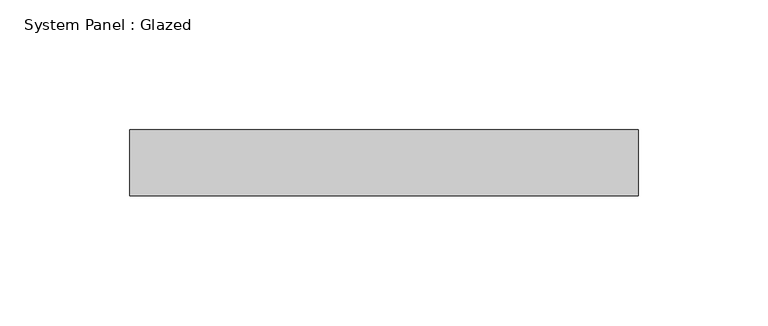
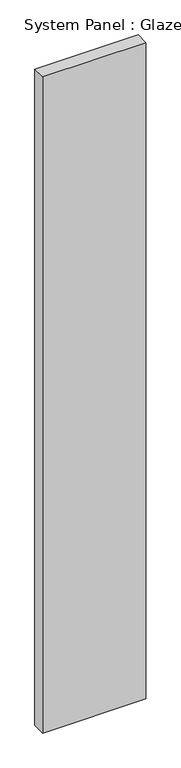
"""IFC4 building model written with IfcOpenShell, lengths in millimetres: plate geometry, System Panel : Glazed."""

from ifc_helpers import new_model, si_unit, origin, origin_with_axes, place, context, project, spatial, polyline, outline, extrude, source, transform, mapped, element, save


def system_panel_glazed_43c0a51f(model_context):
    return source(origin(), model_context, "Body", "SweptSolid", [
        extrude(outline(polyline([(98.0524593, 19.05), (-98.0524593, 19.05), (-98.0524593, 44.45), (98.0524593, 44.45), (98.0524593, 19.05)])), origin_with_axes(), (0.0, 0.0, 1.0), 1319.9815053),
    ])


if __name__ == "__main__":
    model = new_model("IFC4")
    model_context = context("Model", 3, world=origin())
    ifc_project = project(units=[si_unit("LENGTHUNIT", "METRE", prefix="MILLI")], contexts=[model_context])
    site = spatial("IfcSite", under=ifc_project)
    building = spatial("IfcBuilding", under=site)
    placement = place(None, origin())
    system_panel_glazed_shape = system_panel_glazed_43c0a51f(model_context)
    element("IfcPlate", 1, ObjectType="System Panel : Glazed", at=placement, inside=building, context=model_context, shape_type="MappedRepresentation", body=[
        mapped(system_panel_glazed_shape, transform((0.0, 0.0, 0.0), x_axis=(1.0, 0.0, 0.0), y_axis=(0.0, 1.0, 0.0), z_axis=(0.0, 0.0, 1.0))),
    ])
    save(model, "model.ifc")

# Revit data of these elements
# Type "System Panel : Glazed"
#   Construction Type Id = "GSP4R"
#   Analytic Construction = "1/8 in Pilkington single glazing"
#   Visual Light Transmittance = 0.9
#   Solar Heat Gain Coefficient = 0.86
#   Heat Transfer Coefficient (U) = 1.18115 BTU/(h·ft²·°F)
#   Define Thermal Properties by = 1
# Element 1 (IfcPlate, "System Panel : Glazed")
#   Materials on its faces: "Glass"
# Materials
#   "Glass": class "Glass", colour RGB 0 128 192, transparency 0.75, Description = "Soda Lime Glass", Cost = 0
